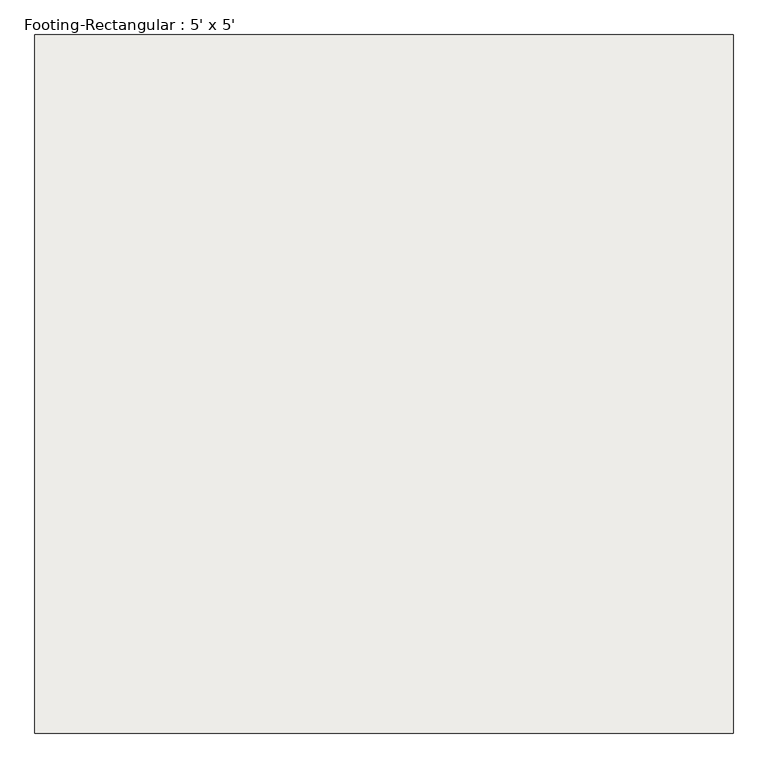
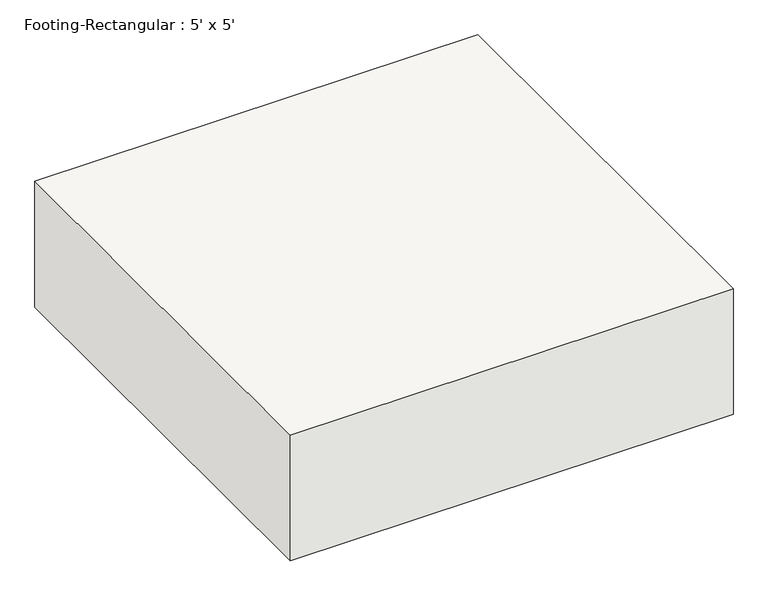
"""IFC4 building model written with IfcOpenShell, lengths in millimetres: slab geometry, Footing-Rectangular : 5' x 5'."""

from ifc_helpers import new_model, si_unit, frame, origin, place, context, project, spatial, polyline, outline, extrude, source, transform, mapped, element, save


def footing_rectangular_5_x_5_df1ede25(model_context):
    return source(origin(), model_context, "Body", "SweptSolid", [
        extrude(outline(polyline([(762.0, 762.0), (762.0, -762.0), (-762.0, -762.0), (-762.0, 762.0), (762.0, 762.0)])), frame((0.0, 0.0, -457.2), z_axis=(0.0, 0.0, 1.0), x_axis=(1.0, 0.0, 0.0)), (0.0, 0.0, 1.0), 457.2),
    ])


if __name__ == "__main__":
    model = new_model("IFC4")
    model_context = context("Model", 3, world=origin())
    ifc_project = project(units=[si_unit("LENGTHUNIT", "METRE", prefix="MILLI")], contexts=[model_context])
    site = spatial("IfcSite", under=ifc_project)
    building = spatial("IfcBuilding", under=site)
    placement = place(None, origin())
    footing_rectangular_5_x_5_shape = footing_rectangular_5_x_5_df1ede25(model_context)
    element("IfcSlab", 1, ObjectType="Footing-Rectangular : 5' x 5'", at=placement, inside=building, context=model_context, shape_type="MappedRepresentation", body=[
        mapped(footing_rectangular_5_x_5_shape, transform((0.0, 0.0, 0.0), x_axis=(1.0, 0.0, 0.0), y_axis=(0.0, 1.0, 0.0), z_axis=(0.0, 0.0, 1.0))),
    ])
    save(model, "model.ifc")

# Revit data of these elements
# Type "Footing-Rectangular : 5' x 5'"
#   Assembly Code = "A1010100"
#   Width = 5' - 0"
#   Length = 5' - 0"
#   Foundation Thickness = 1' - 6"
#   Structural Material [instance default] = Concrete, Cast-in-Place gray
# Element 1 (IfcSlab, "Footing-Rectangular : 5' x 5'")
#   Materials on its faces: "Concrete, Cast-in-Place gray"
# Materials
#   "Concrete, Cast-in-Place gray": class "Concrete", colour RGB 192 192 192, transparency 0, Description = "Cast-in-place concrete", Cost = 0
